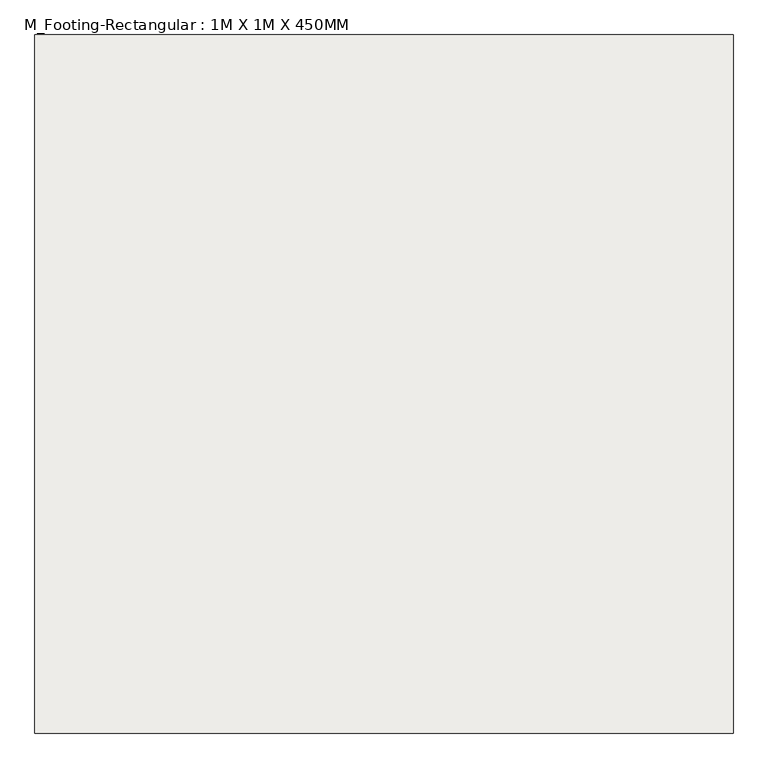
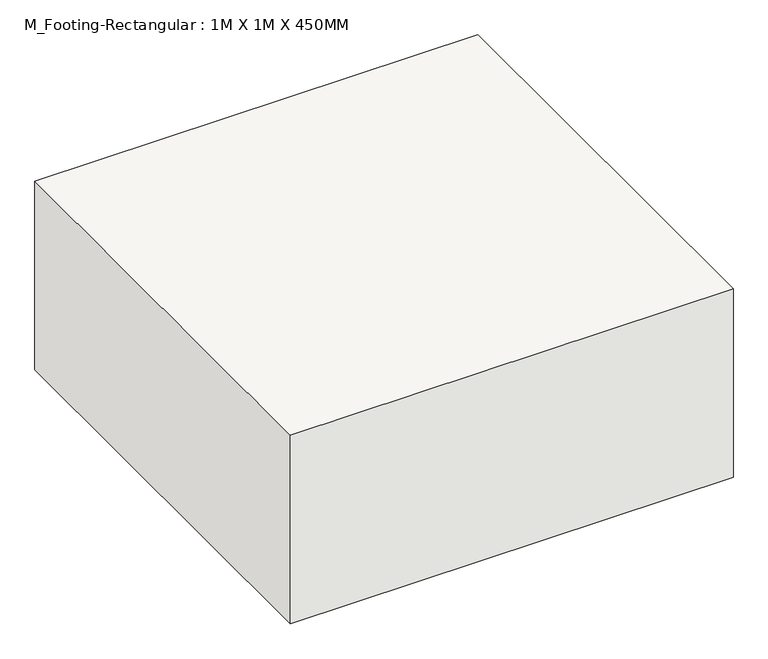
"""IFC4 building model written with IfcOpenShell, lengths in millimetres: slab geometry, M_Footing-Rectangular : 1M X 1M X 450MM."""

from ifc_helpers import new_model, si_unit, frame, origin, place, context, project, spatial, polyline, outline, extrude, source, transform, mapped, element, save


def m_footing_rectangular_1m_x_1m_x_450mm_4c97ae35(model_context):
    return source(origin(), model_context, "Body", "SweptSolid", [
        extrude(outline(polyline([(500.0, 500.0), (500.0, -500.0), (-500.0, -500.0), (-500.0, 500.0), (500.0, 500.0)])), frame((0.0, 0.0, -450.0), z_axis=(0.0, 0.0, 1.0), x_axis=(1.0, 0.0, 0.0)), (0.0, 0.0, 1.0), 450.0),
    ])


if __name__ == "__main__":
    model = new_model("IFC4")
    model_context = context("Model", 3, world=origin())
    ifc_project = project(units=[si_unit("LENGTHUNIT", "METRE", prefix="MILLI")], contexts=[model_context])
    site = spatial("IfcSite", under=ifc_project)
    building = spatial("IfcBuilding", under=site)
    placement = place(None, origin())
    m_footing_rectangular_1m_x_1m_x_450mm_shape = m_footing_rectangular_1m_x_1m_x_450mm_4c97ae35(model_context)
    element("IfcSlab", 1, ObjectType="M_Footing-Rectangular : 1M X 1M X 450MM", at=placement, inside=building, context=model_context, shape_type="MappedRepresentation", body=[
        mapped(m_footing_rectangular_1m_x_1m_x_450mm_shape, transform((0.0, 0.0, 0.0), x_axis=(1.0, 0.0, 0.0), y_axis=(0.0, 1.0, 0.0), z_axis=(0.0, 0.0, 1.0))),
    ])
    save(model, "model.ifc")

# Revit data of these elements
# Type "M_Footing-Rectangular : 1M X 1M X 450MM"
#   Width = 1000 mm
#   Length = 1000 mm
#   Foundation Thickness = 450 mm
#   Structural Material [instance default] = Concrete, Cast-in-Place gray
#   Assembly Code = ""
# Element 1 (IfcSlab, "M_Footing-Rectangular : 1M X 1M X 450MM")
#   Materials on its faces: "Concrete, Cast-in-Place gray"
# Materials
#   "Concrete, Cast-in-Place gray": class "Concrete", colour RGB 192 192 192, transparency 0, Description = "Cast-in-place concrete", Cost = 0
